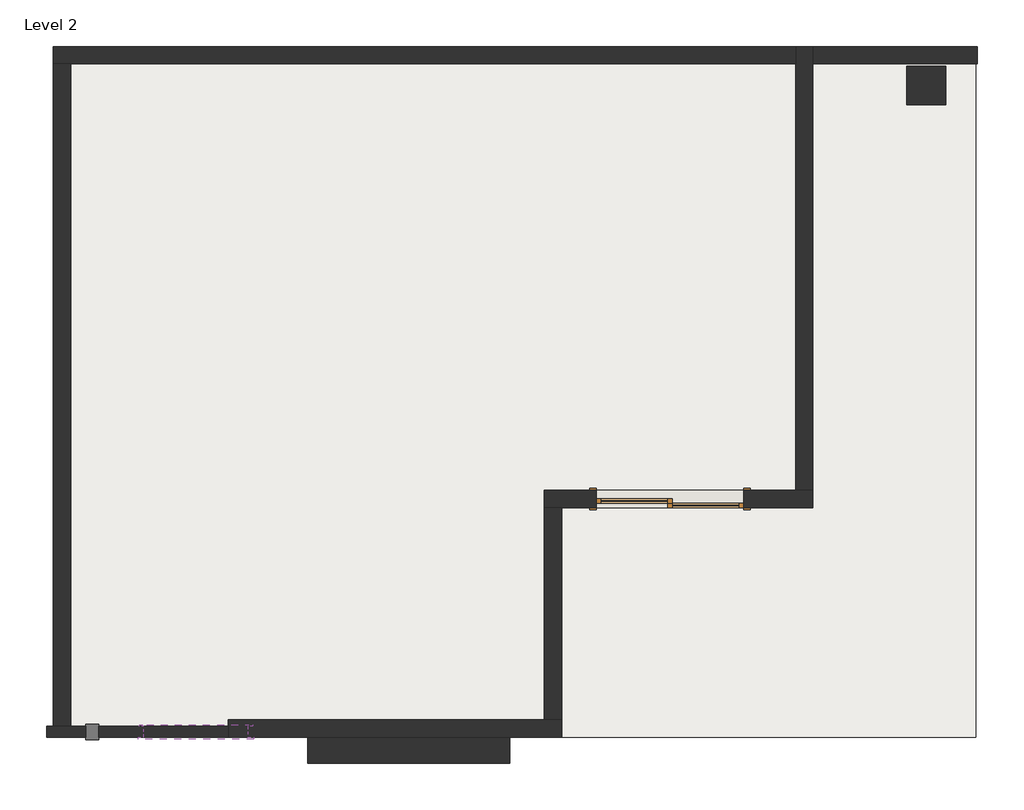
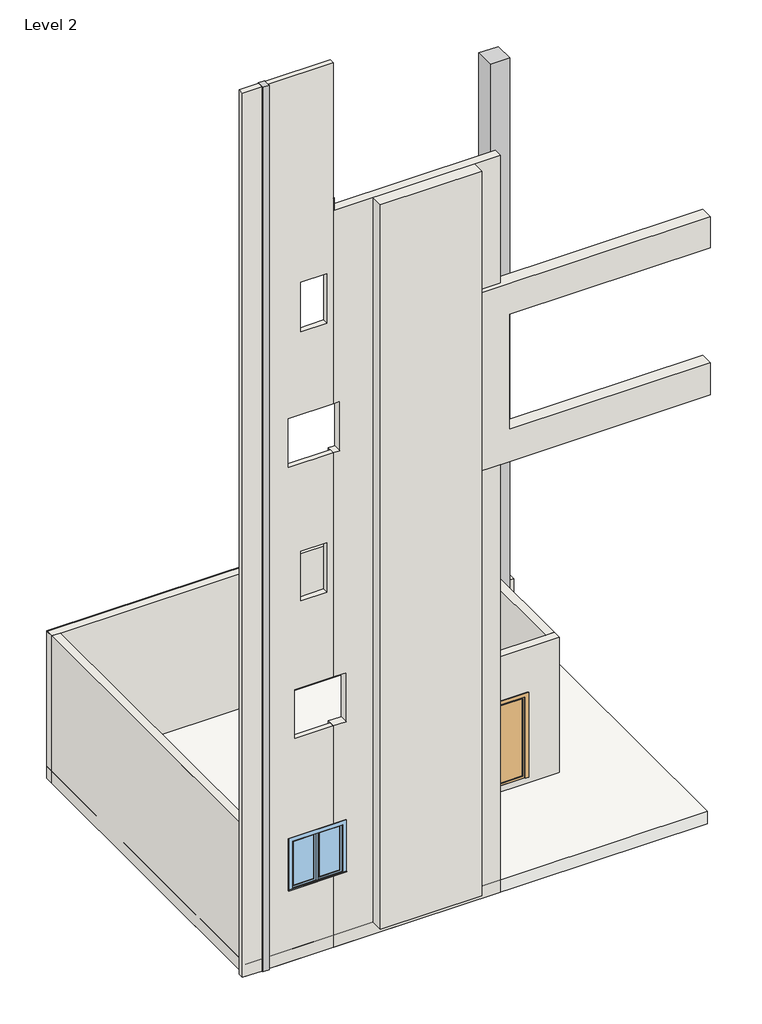
# One storey, incomplete: 9 walls, 1 column, 1 door, 1 proxy, 1 roof, 1 window.
"""IFC4 building model written with IfcOpenShell, lengths in millimetres."""

from ifc_helpers import new_model, si_unit, frame, origin, place, context, project, spatial, polyline, outline, extrude, faceted_brep, transform, mapped, element, save
from components import column_5762f69e, door_076b30e0, walls_1_walls_1_998562f7, window_40d2abec

model = new_model("IFC4")

# Units and contexts
model_context = context("Model", 3, world=origin())
ifc_project = project(units=[si_unit("LENGTHUNIT", "METRE", prefix="MILLI")], contexts=[model_context])

# Site, building, storey
site = spatial("IfcSite", under=ifc_project)
building = spatial("IfcBuilding", under=site)
storey = spatial("IfcBuildingStorey", under=building, Name="Level 2", Elevation=3657.6)

# Proxy
placement = place(None, origin())
element("IfcBuildingElementProxy", 1, Name="Reveal", ObjectType="Reveal", at=placement, inside=storey, context=model_context, shape_type="SweptSolid", body=[
    extrude(outline(polyline([(-13834.7304753, 2825.1497737), (-13834.7304753, 3008.0297737), (-13682.3304753, 3008.0297737), (-13682.3304753, 2825.1497737), (-13834.7304753, 2825.1497737)])), frame((0.0, 0.0, 3657.6), z_axis=(0.0, 0.0, 1.0), x_axis=(1.0, 0.0, 0.0)), (0.0, 0.0, 1.0), 21945.6),
])

# Column
column_shape = column_5762f69e(model_context)
element("IfcColumn", 2, ObjectType="Rectangular Column : 18\" x 18\"", at=placement, inside=storey, context=model_context, shape_type="MappedRepresentation", body=[
    mapped(column_shape, transform((-3970.1492777, 10501.0297737, 0.0), x_axis=(1.0, 0.0, 0.0), y_axis=(0.0, 1.0, 0.0), z_axis=(0.0, 0.0, 1.0))),
])

# Door
door_shape = door_076b30e0(model_context)
element("IfcDoor", 3, ObjectType="Door-Double-Sliding : 68\" x 80\"", at=placement, inside=storey, context=model_context, shape_type="MappedRepresentation", body=[
    mapped(door_shape, transform((-6976.7304753, 5777.4732783, 4114.8), x_axis=(-1.0, 0.0, 0.0), y_axis=(0.0, -1.0, 0.0), z_axis=(0.0, 0.0, 1.0))),
])

# Roof
element("IfcRoof", 4, ObjectType="Generic - 12\"", at=placement, inside=storey, context=model_context, shape_type="SweptSolid", body=[
    extrude(outline(polyline([(-14209.7864811, 10932.8297737), (-3389.3864811, 10932.8297737), (-3389.3864811, 2855.6297737), (-14209.7864811, 2855.6297737), (-14209.7864811, 10932.8297737)])), frame((0.0, 0.0, 3657.6), z_axis=(0.0, 0.0, 1.0), x_axis=(1.0, 0.0, 0.0)), (0.0, 0.0, 1.0), 304.8),
])

# Walls
element("IfcWall", 5, ObjectType="Generic - 5\"", at=placement, inside=storey, context=model_context, shape_type="Brep", body=[
    faceted_brep([(-14291.9304753, 2982.6297737, 3657.6), (-14291.9304753, 2982.6297737, 25603.2), (-13834.7304753, 2982.6297737, 25603.2), (-13834.7304753, 2982.6297737, 3657.6), (-14009.4992777, 2982.6297737, 3657.6), (-14212.6992777, 2982.6297737, 3657.6), (-14291.9304753, 2855.6297737, 25603.2), (-14291.9304753, 2855.6297737, 3657.6), (-13834.7304753, 2855.6297737, 3657.6), (-13834.7304753, 2855.6297737, 25603.2)], [[[0, 1, 2, 3, 4, 5]], [[6, 7, 8, 9]], [[7, 0, 5, 4, 3, 8]], [[1, 0, 7, 6]], [[1, 6, 9, 2]], [[3, 2, 9, 8]]]),
    faceted_brep([(-12158.3304753, 2982.6297737, 5439.2953607), (-12158.3304753, 2982.6297737, 3657.6), (-13682.3304753, 2982.6297737, 3657.6), (-13682.3304753, 2982.6297737, 25603.2), (-12158.3304753, 2982.6297737, 25603.2), (-12158.3304753, 2982.6297737, 17150.104066), (-13225.1304753, 2982.6297737, 17150.104066), (-13225.1304753, 2982.6297737, 15930.904066), (-12158.3304753, 2982.6297737, 15930.904066), (-12158.3304753, 2982.6297737, 10370.4437858), (-13072.7304753, 2982.6297737, 10370.4437858), (-13072.7304753, 2982.6297737, 9151.2437858), (-12158.3304753, 2982.6297737, 9151.2437858), (-12158.3304753, 2982.6297737, 6658.4953607), (-13148.9304753, 2982.6297737, 6658.4953607), (-13148.9304753, 2982.6297737, 5439.2953607), (-12310.7304753, 2982.6297737, 12527.8331892), (-12310.7304753, 2982.6297737, 13747.0331892), (-12920.3304753, 2982.6297737, 13747.0331892), (-12920.3304753, 2982.6297737, 12527.8331892), (-12310.7304753, 2982.6297737, 19202.4), (-12310.7304753, 2982.6297737, 20421.6), (-12920.3304753, 2982.6297737, 20421.6), (-12920.3304753, 2982.6297737, 19202.4), (-12158.3304753, 2855.6297737, 3657.6), (-12158.3304753, 2855.6297737, 5439.2953607), (-13148.9304753, 2855.6297737, 5439.2953607), (-13148.9304753, 2855.6297737, 6658.4953607), (-12158.3304753, 2855.6297737, 6658.4953607), (-12158.3304753, 2855.6297737, 9151.2437858), (-13072.7304753, 2855.6297737, 9151.2437858), (-13072.7304753, 2855.6297737, 10370.4437858), (-12158.3304753, 2855.6297737, 10370.4437858), (-12158.3304753, 2855.6297737, 15930.904066), (-13225.1304753, 2855.6297737, 15930.904066), (-13225.1304753, 2855.6297737, 17150.104066), (-12158.3304753, 2855.6297737, 17150.104066), (-12158.3304753, 2855.6297737, 22250.4), (-12158.3304753, 2855.6297737, 25603.2), (-13682.3304753, 2855.6297737, 25603.2), (-13682.3304753, 2855.6297737, 3657.6), (-12310.7304753, 2855.6297737, 13747.0331892), (-12310.7304753, 2855.6297737, 12527.8331892), (-12920.3304753, 2855.6297737, 12527.8331892), (-12920.3304753, 2855.6297737, 13747.0331892), (-12310.7304753, 2855.6297737, 20421.6), (-12310.7304753, 2855.6297737, 19202.4), (-12920.3304753, 2855.6297737, 19202.4), (-12920.3304753, 2855.6297737, 20421.6)], [[[0, 1, 2, 3, 4, 5, 6, 7, 8, 9, 10, 11, 12, 13, 14, 15], [16, 17, 18, 19], [20, 21, 22, 23]], [[24, 25, 26, 27, 28, 29, 30, 31, 32, 33, 34, 35, 36, 37, 38, 39, 40], [41, 42, 43, 44], [45, 46, 47, 48]], [[1, 24, 40, 2]], [[38, 4, 3, 39]], [[4, 38, 37, 36, 5]], [[24, 1, 0, 25]], [[28, 13, 12, 29]], [[32, 9, 8, 33]], [[3, 2, 40, 39]], [[14, 27, 26, 15]], [[15, 26, 25, 0]], [[27, 14, 13, 28]], [[10, 31, 30, 11]], [[11, 30, 29, 12]], [[31, 10, 9, 32]], [[6, 35, 34, 7]], [[7, 34, 33, 8]], [[35, 6, 5, 36]], [[42, 41, 17, 16]], [[43, 42, 16, 19]], [[44, 43, 19, 18]], [[41, 44, 18, 17]], [[46, 45, 21, 20]], [[47, 46, 20, 23]], [[48, 47, 23, 22]], [[45, 48, 22, 21]]]),
])
element("IfcWall", 6, ObjectType="Generic - 8\"", at=placement, inside=storey, context=model_context, shape_type="Brep", body=[
    faceted_brep([(-5300.3304753, 5752.0732783, 3657.6), (-5503.5304753, 5752.0732783, 3657.6), (-8449.9304753, 5752.0732783, 3657.6), (-8449.9304753, 5752.0732783, 7315.2), (-5503.5304753, 5752.0732783, 7315.2), (-5300.3304753, 5752.0732783, 7315.2), (-6113.1304753, 5752.0732783, 6146.8), (-7840.3304753, 5752.0732783, 6146.8), (-7840.3304753, 5752.0732783, 4114.8), (-6113.1304753, 5752.0732783, 4114.8), (-5300.3304753, 5548.8732783, 3657.6), (-5300.3304753, 5548.8732783, 7315.2), (-8246.7304753, 5548.8732783, 7315.2), (-8449.9304753, 5548.8732783, 7315.2), (-8449.9304753, 5548.8732783, 3657.6), (-8246.7304753, 5548.8732783, 3657.6), (-6113.1304753, 5548.8732783, 6146.8), (-6113.1304753, 5548.8732783, 4114.8), (-7840.3304753, 5548.8732783, 4114.8), (-7840.3304753, 5548.8732783, 6146.8)], [[[0, 1, 2, 3, 4, 5], [6, 7, 8, 9]], [[10, 11, 12, 13, 14, 15], [16, 17, 18, 19]], [[2, 1, 0, 10, 15, 14]], [[3, 2, 14, 13]], [[0, 5, 11, 10]], [[5, 4, 3, 13, 12, 11]], [[17, 16, 6, 9]], [[18, 17, 9, 8]], [[19, 18, 8, 7]], [[16, 19, 7, 6]]]),
])
element("IfcWall", 7, ObjectType="Generic - 8\"", at=placement, inside=storey, context=model_context, shape_type="SweptSolid", body=[
    extrude(outline(polyline([(-8449.9304753, 3058.8297737), (-8449.9304753, 5548.8732783), (-8246.7304753, 5548.8732783), (-8246.7304753, 3058.8297737), (-8449.9304753, 3058.8297737)])), frame((0.0, 0.0, 3657.6), z_axis=(0.0, 0.0, 1.0), x_axis=(1.0, 0.0, 0.0)), (0.0, 0.0, 1.0), 3657.6),
])
element("IfcWall", 8, ObjectType="Generic - 8\"", at=placement, inside=storey, context=model_context, shape_type="Brep", body=[
    faceted_brep([(-5300.3304753, 5752.0732783, 3657.6), (-5300.3304753, 10958.2297737, 3657.6), (-5300.3304753, 10958.2297737, 3944.4125244), (-5300.3304753, 10958.2297737, 4933.2392493), (-5300.3304753, 10958.2297737, 7315.2), (-5300.3304753, 10932.8297737, 7315.2), (-5300.3304753, 5752.0732783, 7315.2), (-5503.5304753, 5752.0732783, 3657.6), (-5503.5304753, 5752.0732783, 7315.2), (-5503.5304753, 10755.0297737, 7315.2), (-5503.5304753, 10932.8297737, 7315.2), (-5503.5304753, 10958.2297737, 7315.2), (-5503.5304753, 10958.2297737, 3657.6), (-5503.5304753, 10755.0297737, 3657.6)], [[[0, 1, 2, 3, 4, 5, 6]], [[7, 8, 9, 10, 11, 12, 13]], [[1, 0, 7, 13, 12]], [[0, 6, 8, 7]], [[5, 4, 11, 10]], [[6, 5, 10, 9, 8]], [[1, 12, 11, 4, 3, 2]]]),
])
element("IfcWall", 9, ObjectType="Generic - 8\"", at=placement, inside=storey, context=model_context, shape_type="Brep", body=[
    faceted_brep([(-5503.5304753, 10958.2297737, 7315.2), (-5503.5304753, 10958.2297737, 3657.6), (-14212.6992777, 10958.2297737, 3657.6), (-14212.6992777, 10958.2297737, 7315.2), (-14209.7864811, 10958.2297737, 7315.2), (-5503.5304753, 10755.0297737, 3657.6), (-5503.5304753, 10755.0297737, 7315.2), (-14009.4992777, 10755.0297737, 7315.2), (-14209.7864811, 10755.0297737, 7315.2), (-14212.6992777, 10755.0297737, 7315.2), (-14212.6992777, 10755.0297737, 3657.6), (-14009.4992777, 10755.0297737, 3657.6), (-14212.6992777, 10932.8297737, 7315.2), (-14209.7864811, 10932.8297737, 7315.2), (-5503.5304753, 10932.8297737, 7315.2)], [[[0, 1, 2, 3, 4]], [[5, 6, 7, 8, 9, 10, 11]], [[2, 1, 5, 11, 10]], [[3, 2, 10, 9, 12]], [[12, 9, 8, 13]], [[0, 4, 13, 14]], [[4, 3, 12, 13]], [[8, 7, 6, 14, 13]], [[0, 14, 6, 5, 1]]]),
])
element("IfcWall", 10, ObjectType="Generic - 8\"", at=placement, inside=storey, context=model_context, shape_type="Brep", body=[
    faceted_brep([(-14212.6992777, 10755.0297737, 3657.6), (-14212.6992777, 2982.6297737, 3657.6), (-14212.6992777, 2982.6297737, 7315.2), (-14212.6992777, 3058.8297737, 7315.2), (-14212.6992777, 10755.0297737, 7315.2), (-14009.4992777, 10755.0297737, 3657.6), (-14009.4992777, 10755.0297737, 7315.2), (-14009.4992777, 3058.8297737, 7315.2), (-14009.4992777, 2982.6297737, 7315.2), (-14009.4992777, 2982.6297737, 3657.6), (-14209.7864811, 10755.0297737, 7315.2), (-14209.7864811, 3058.8297737, 7315.2), (-14209.7864811, 2982.6297737, 7315.2)], [[[0, 1, 2, 3, 4]], [[5, 6, 7, 8, 9]], [[1, 0, 5, 9]], [[0, 4, 10, 6, 5]], [[4, 3, 11, 10]], [[12, 8, 7, 11]], [[3, 2, 12, 11]], [[11, 7, 6, 10]], [[2, 1, 9, 8, 12]]]),
])
element("IfcWall", 11, ObjectType="Generic - 8\"", at=placement, inside=storey, context=model_context, shape_type="Brep", body=[
    faceted_brep([(-12158.3304753, 2855.6297737, 3657.6), (-8246.7304753, 2855.6297737, 3657.6), (-8246.7304753, 2855.6297737, 21945.6), (-12139.2804753, 2855.6297737, 21945.6), (-12139.2804753, 2855.6297737, 22250.4), (-12158.3304753, 2855.6297737, 22250.4), (-12158.3304753, 2855.6297737, 17150.104066), (-12005.9304753, 2855.6297737, 17150.104066), (-12005.9304753, 2855.6297737, 15930.904066), (-12158.3304753, 2855.6297737, 15930.904066), (-12158.3304753, 2855.6297737, 10370.4437858), (-11853.5304753, 2855.6297737, 10370.4437858), (-11853.5304753, 2855.6297737, 9151.2437858), (-12158.3304753, 2855.6297737, 9151.2437858), (-12158.3304753, 2855.6297737, 6658.4953607), (-11929.7304753, 2855.6297737, 6658.4953607), (-11929.7304753, 2855.6297737, 5439.2953607), (-12158.3304753, 2855.6297737, 5439.2953607), (-8246.7304753, 3058.8297737, 3657.6), (-8449.9304753, 3058.8297737, 3657.6), (-12158.3304753, 3058.8297737, 3657.6), (-12158.3304753, 3058.8297737, 5439.2953607), (-11929.7304753, 3058.8297737, 5439.2953607), (-11929.7304753, 3058.8297737, 6658.4953607), (-12158.3304753, 3058.8297737, 6658.4953607), (-12158.3304753, 3058.8297737, 9151.2437858), (-11853.5304753, 3058.8297737, 9151.2437858), (-11853.5304753, 3058.8297737, 10370.4437858), (-12158.3304753, 3058.8297737, 10370.4437858), (-12158.3304753, 3058.8297737, 15930.904066), (-12005.9304753, 3058.8297737, 15930.904066), (-12005.9304753, 3058.8297737, 17150.104066), (-12158.3304753, 3058.8297737, 17150.104066), (-12158.3304753, 3058.8297737, 22250.4), (-12139.2804753, 3058.8297737, 22250.4), (-12139.2804753, 3058.8297737, 21945.6), (-8449.9304753, 3058.8297737, 21945.6), (-8246.7304753, 3058.8297737, 21945.6), (-8246.7304753, 3058.8297737, 18288.0), (-8246.7304753, 3058.8297737, 14630.4), (-8246.7304753, 3058.8297737, 10972.8), (-8246.7304753, 3058.8297737, 7315.2), (-12158.3304753, 2982.6297737, 3657.6), (-12158.3304753, 2982.6297737, 17150.104066), (-12158.3304753, 2982.6297737, 5439.2953607), (-12158.3304753, 2982.6297737, 6658.4953607), (-12158.3304753, 2982.6297737, 9151.2437858), (-12158.3304753, 2982.6297737, 10370.4437858), (-12158.3304753, 2982.6297737, 15930.904066)], [[[0, 1, 2, 3, 4, 5, 6, 7, 8, 9, 10, 11, 12, 13, 14, 15, 16, 17]], [[18, 19, 20, 21, 22, 23, 24, 25, 26, 27, 28, 29, 30, 31, 32, 33, 34, 35, 36, 37, 38, 39, 40, 41]], [[1, 0, 42, 20, 19, 18]], [[5, 33, 32, 43, 6]], [[20, 42, 0, 17, 44, 21]], [[24, 45, 14, 13, 46, 25]], [[28, 47, 10, 9, 48, 29]], [[1, 18, 41, 40, 39, 38, 37, 2]], [[33, 5, 4, 34]], [[34, 4, 3, 35]], [[3, 2, 37, 36, 35]], [[16, 22, 21, 44, 17]], [[22, 16, 15, 23]], [[23, 15, 14, 45, 24]], [[12, 26, 25, 46, 13]], [[26, 12, 11, 27]], [[27, 11, 10, 47, 28]], [[8, 30, 29, 48, 9]], [[30, 8, 7, 31]], [[31, 7, 6, 43, 32]]]),
])
element("IfcWall", 12, ObjectType="Generic - 8\"", at=placement, inside=storey, context=model_context, shape_type="SweptSolid", body=[
    extrude(outline(polyline([(-3369.9304753, 10755.0297737), (-5300.3304753, 10755.0297737), (-5300.3304753, 10958.2297737), (-3369.9304753, 10958.2297737), (-3369.9304753, 10755.0297737)])), frame((0.0, 0.0, 3944.4125244), z_axis=(0.0, 0.0, 1.0), x_axis=(1.0, 0.0, 0.0)), (0.0, 0.0, 1.0), 988.8267249),
])
walls_1_walls_1_shape = walls_1_walls_1_998562f7(model_context)
element("IfcWall", 13, ObjectType="Walls 1 : Walls 1", at=placement, inside=storey, context=model_context, shape_type="MappedRepresentation", body=[
    mapped(walls_1_walls_1_shape, transform((0.0, 0.0, 0.0), x_axis=(1.0, 0.0, 0.0), y_axis=(0.0, 1.0, 0.0), z_axis=(0.0, 0.0, 1.0))),
])

# Window
window_shape = window_40d2abec(model_context)
element("IfcWindow", 14, ObjectType="Casement Dbl with Trim.0001 : 48\" x 48\"", at=placement, inside=storey, context=model_context, shape_type="MappedRepresentation", body=[
    mapped(window_shape, transform((-12539.3304753, 2938.1797737, 4524.8953607), x_axis=(-1.0, 0.0, 0.0), y_axis=(0.0, -1.0, 0.0), z_axis=(0.0, 0.0, 1.0))),
])

save(model, "model.ifc")

# Revit data of these elements
# Type "Rectangular Column : 18\" x 18\""
#   Assembly Code = "B1010200"
#   Depth = 1' - 6"
#   Offset Base = 0' - 0"
#   Offset Top = 0' - 0"
#   Width = 1' - 6"
#   Material = none
# Type "Door-Double-Sliding : 68\" x 80\""
#   Type Mark = "8"
#   Construction Type Id = "opn-d45"
#   Assembly Code = "C1020"
#   Analytic Construction = "Wood frame, double glass door "
#   Thickness = 0' - 2"
#   Thermal Resistance (R) = 1.8150 (h·ft²·°F)/BTU
#   Heat Transfer Coefficient (U) = 0.5510 BTU/(h·ft²·°F)
#   Height = 6' - 8"
#   Rail Width = 0' - 2"
#   Stiles = 0' - 2"
#   Trim Projection Ext = 0' - 1"
#   Trim Projection Int = 0' - 1"
#   Trim Width = 0' - 3"
#   Width = 5' - 8"
#   Define Thermal Properties by = 1
#   Glazing = Glass
#   Panel Material = Wood - Birch - Solid Stained Light Low Gloss
#   Trim Material = Paint - Sienna
#   Visual Light Transmittance = 0
#   Solar Heat Gain Coefficient = 0
#   Function = (empty or 0)
#   Wall Closure = (empty or 0)
# Type "Generic - 12\""
#   Assembly Code = "B1020"
#   Layers, outside or top first: 1' - 0" no material (function 1)
# Type "Generic - 5\""
#   Assembly Code = "B2010"
#   Layers, outside or top first: 0' - 5" no material (function 1)
# Type "Generic - 8\""
#   Assembly Code = "B2010"
#   Layers, outside or top first: 0' - 8" no material (function 1)
# Type "Casement Dbl with Trim.0001 : 48\" x 48\""
#   Type Mark = "10"
#   Construction Type Id = "GSP4R"
#   Assembly Code = "B2020100"
#   Analytic Construction = "1/8 in Pilkington single glazing"
#   Visual Light Transmittance = 0.9
#   Solar Heat Gain Coefficient = 0.78
#   Heat Transfer Coefficient (U) = 0.6496 BTU/(h·ft²·°F)
#   Height = 4' - 0"
#   Default Sill Height = 3' - 0"
#   Trim Projection - Ext. = 0' - 0 1/2"
#   Trim Projection - Int. = 0' - 0 3/4"
#   Trim Width - Exterior = 0' - 3 1/2"
#   Trim Width - Interior = 0' - 3 1/2"
#   Width = 4' - 0"
#   Window Inset = 0' - 0 3/4"
#   Define Thermal Properties by = 1
#   Glass Pane Material = Glass
#   Sash Material = Sash
#   Trim Exterior Material = Trim
#   Trim Interior Material = Trim
#   Wall Closure = (empty or 0)
# Element 2 (IfcColumn, "Rectangular Column : 18\" x 18\"")
#   Phase Created = New Construction
# Element 3 (IfcDoor, "Door-Double-Sliding : 68\" x 80\"")
#   Phase Created = New Construction
#   Materials on its faces: "Paint - Sienna", "Wood - Birch - Solid Stained Light Low Gloss", "Glass"
# Element 4 (IfcRoof, "Generic - 12\"")
#   built-in parameter 1001705 = 13 (stored number, unit not read)
#   built-in parameter 1001710 = 33615
#   Phase Created = New Construction
#   Materials on its faces: "Default Roof"
# Element 5 (IfcWall, "Generic - 5\"")
#   Top Offset = 60' - 0"
#   Base Offset = 0' - 0"
#   wall height = 72' - 0"
#   Phase Created = New Construction
#   Base Constraint = Level 2
#   Top Constraint = Level 3
#   Materials on its faces: "Default Wall"
# Elements 6, 7, 8, 9, 10 (IfcWall, "Generic - 8\"")
#   Top Offset = 0' - 0"
#   Base Offset = 0' - 0"
#   Unconnected Height = 12' - 0"
#   wall height = 12' - 0"
#   Phase Created = New Construction
#   Base Constraint = Level 2
#   Materials on its faces: "Default Wall"
# Element 11 (IfcWall, "Generic - 8\"")
#   Top Offset = 0' - 0"
#   Base Offset = 0' - 0"
#   Unconnected Height = 61' - 0"
#   wall height = 61' - 0"
#   Phase Created = New Construction
#   Base Constraint = Level 2
#   Materials on its faces: "Default Wall"
# Element 12 (IfcWall, "Generic - 8\"")
#   built-in parameter 1001111 = 0' - 11.29183"
#   Top Offset = 0' - 0"
#   Base Offset = 0' - 11.29183"
#   Unconnected Height = 3' - 2.93019"
#   wall height = 3' - 2.93019"
#   Phase Created = New Construction
#   Base Constraint = Level 2
#   Materials on its faces: "Default Wall"
# Element 13 (IfcWall, "Walls 1 : Walls 1")
#   Phase Created = New Construction
#   Materials on its faces: "Default Wall"
# Element 14 (IfcWindow, "Casement Dbl with Trim.0001 : 48\" x 48\"")
#   Mark = "3"
#   Phase Created = New Construction
#   Materials on its faces: "Sash", "Trim", "Glass"
# Materials
#   "Glass": class "Glass", colour RGB 0 128 192, transparency 0.75, Description = "Soda Lime Glass", Cost = 0
#   "Wood - Birch - Solid Stained Light Low Gloss": class "Wood", colour RGB 210 159 95, transparency 0, Cost = 0
#   "Paint - Sienna": colour RGB 118 70 51, transparency 0, Cost = 0
#   "Sash": class "Wood", colour RGB 224 178 126, transparency 0
#   "Trim": class "Wood", colour RGB 224 178 126, transparency 0
#   "Default Roof": colour RGB 88 101 114, transparency 0
#   "Default Wall": colour RGB 128 128 128, transparency 0
